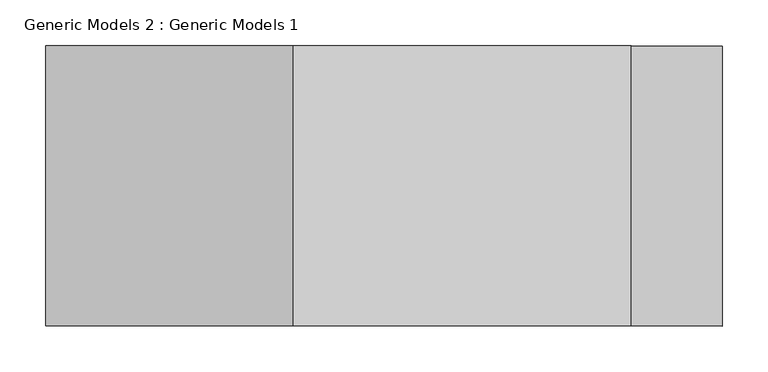
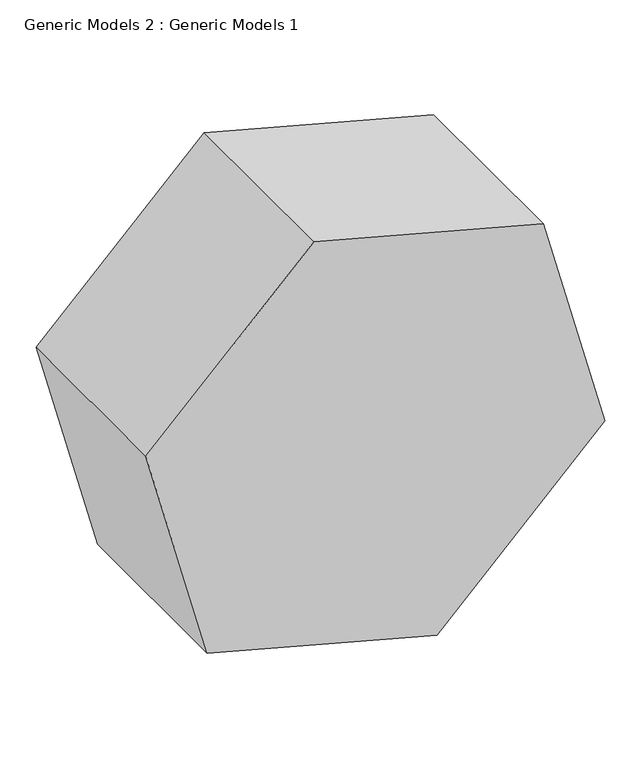
"""IFC4 building model written with IfcOpenShell, lengths in millimetres: proxy geometry, Generic Models 2 : Generic Models 1."""

from ifc_helpers import new_model, si_unit, frame, origin, place, context, project, spatial, polyline, outline, extrude, source, transform, mapped, element, save


def generic_models_2_generic_models_1_372cb617(model_context):
    return source(origin(), model_context, "Body", "SweptSolid", [
        extrude(outline(polyline([(904.7566299, -9035.0070438), (1003.366686, -9403.0247836), (733.9590024, -9672.4324672), (365.9412626, -9573.822411), (267.3312064, -9205.8046712), (536.73889, -8936.3969876), (904.7566299, -9035.0070438)])), frame((0.0, -9086.6225464, 0.0), z_axis=(0.0, 1.0, 0.0), x_axis=(0.0, 0.0, 1.0)), (0.0, 0.0, 1.0), 304.8),
    ])


if __name__ == "__main__":
    model = new_model("IFC4")
    model_context = context("Model", 3, world=origin())
    ifc_project = project(units=[si_unit("LENGTHUNIT", "METRE", prefix="MILLI")], contexts=[model_context])
    site = spatial("IfcSite", under=ifc_project)
    building = spatial("IfcBuilding", under=site)
    placement = place(None, origin())
    generic_models_2_generic_models_1_shape = generic_models_2_generic_models_1_372cb617(model_context)
    element("IfcBuildingElementProxy", 1, Name="Generic Models 2 : Generic Models 1", ObjectType="Generic Models 2 : Generic Models 1", at=placement, inside=building, context=model_context, shape_type="MappedRepresentation", body=[
        mapped(generic_models_2_generic_models_1_shape, transform((0.0, 0.0, 0.0), x_axis=(1.0, 0.0, 0.0), y_axis=(0.0, 1.0, 0.0), z_axis=(0.0, 0.0, 1.0))),
    ])
    save(model, "model.ifc")

# Revit data of these elements
# Element 1 (IfcBuildingElementProxy, "Generic Models 2 : Generic Models 1")
#   Materials on its faces: "Brick, Common"
# Materials
#   "Brick, Common": class "Masonry", colour RGB 170 98 104, transparency 0, Description = "Common brick", Cost = 0
